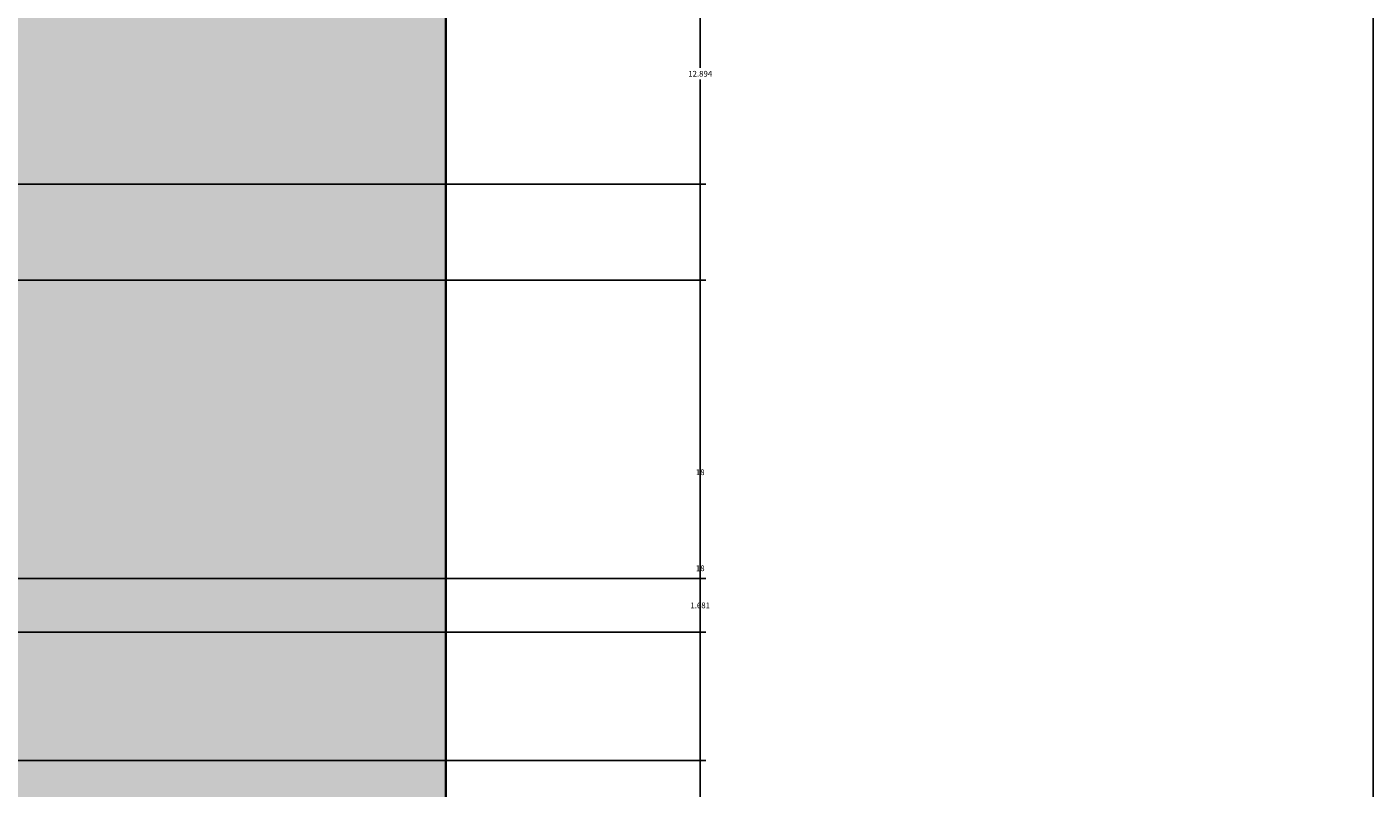
# Model space of a CAD drawing. Units: inches. Extents: x 4508 to 4723, y 847 to 1020.
# Tile 24 of 32: x 4681 to 4723, y 886 to 910. Entities that reach past the tile are written whole.
import ezdxf

# ---------------------------------------------------------------- set-up
doc = ezdxf.new("R2010")
doc.units = ezdxf.units.IN
for name, color, linetype, lineweight in [('A-ANNO-DIMS', 2, 'Continuous', 18), ('A-ANNO-TTLB', 7, 'Continuous', 25), ('A-WALL', 7, 'Continuous', 35), ('A-WALL-PATT', 254, 'Continuous', 13)]:
    doc.layers.add(name, color=color, linetype=linetype, lineweight=lineweight)
doc.styles.get("Standard").update_dxf_attribs({"font": 'arial.ttf'})
doc.dimstyles.get("Standard").update_dxf_attribs({"dimtxt": 0.18, "dimasz": 0.18, "dimexe": 0.18, "dimexo": 0.0625, "dimgap": 0.09, "dimtad": 0, "dimtih": 1, "dimtoh": 1, "dimdec": 4, "dimzin": 0, "dimdsep": 46, "dimtxsty": 'Standard', "dimcen": 0.09, "dimadec": 0, "dimazin": 0, "dimtfac": 1, "dimtdec": 4, "dimtofl": 0, "dimtmove": 0, "dimatfit": 3, "dimfxl": 1, "dimtolj": 1, "dimtzin": 0, "dimarcsym": 0})

# ---------------------------------------------------------------- blocks, each defined once
blk = doc.blocks.new('*D13')
at = {"layer": 'A-ANNO-DIMS', "color": 0, "lineweight": -2, "transparency": 16777216}
for p, q in [((4669.325, 973.916), (4669.325, 866.617)), ((4689.994, 874.684), (4689.994, 866.617)), ((4669.505, 866.797), (4679.264, 866.797)), ((4689.814, 866.797), (4680.054, 866.797))]:
    blk.add_line(p, q, dxfattribs=at)
at = {"layer": 'A-ANNO-DIMS', "color": 0, "lineweight": 9, "transparency": 16777216}
for points in [[(4669.505, 866.827), (4669.505, 866.767), (4669.325, 866.797)], [(4689.814, 866.827), (4689.814, 866.767), (4689.994, 866.797)]]:
    blk.add_solid(points, dxfattribs=at)
at = {"layer": 'Defpoints', "color": 0, "lineweight": 9, "transparency": 16777216}
for p in [(4669.325, 973.978), (4689.994, 874.747), (4689.994, 866.797)]:
    blk.add_point(p, dxfattribs=at)
at = {"layer": 'A-ANNO-DIMS', "color": 0, "transparency": 16777216, "insert": (4679.659, 866.797), "char_height": 0.18, "attachment_point": 5}
blk.add_mtext('\\A1;20.67', dxfattribs=at)
blk = doc.blocks.new('*D18')
at = {"layer": 'A-ANNO-DIMS', "color": 0, "lineweight": -2, "transparency": 16777216}
for p, q in [((4671.119, 901.747), (4702.124, 901.747)), ((4701.944, 901.567), (4701.944, 892.929)), ((4701.944, 883.927), (4701.944, 892.565)), ((4671.869, 883.747), (4702.124, 883.747))]:
    blk.add_line(p, q, dxfattribs=at)
at = {"layer": 'A-ANNO-DIMS', "color": 0, "lineweight": 9, "transparency": 16777216}
for points in [[(4701.914, 901.567), (4701.974, 901.567), (4701.944, 901.747)], [(4701.914, 883.927), (4701.974, 883.927), (4701.944, 883.747)]]:
    blk.add_solid(points, dxfattribs=at)
at = {"layer": 'Defpoints', "color": 0, "lineweight": 9, "transparency": 16777216}
for p in [(4671.056, 901.747), (4701.944, 901.747), (4671.806, 883.747)]:
    blk.add_point(p, dxfattribs=at)
at = {"layer": 'A-ANNO-DIMS', "color": 0, "transparency": 16777216, "insert": (4701.944, 892.747), "char_height": 0.18, "attachment_point": 5}
blk.add_mtext('\\A1;18', dxfattribs=at)
blk = doc.blocks.new('*D19')
at = {"layer": 'A-ANNO-DIMS', "color": 0, "lineweight": -2, "transparency": 16777216}
for p, q in [((4662.233, 914.641), (4702.124, 914.641)), ((4701.944, 914.461), (4701.944, 908.376)), ((4701.944, 901.927), (4701.944, 908.012)), ((4671.119, 901.747), (4702.124, 901.747))]:
    blk.add_line(p, q, dxfattribs=at)
at = {"layer": 'A-ANNO-DIMS', "color": 0, "lineweight": 9, "transparency": 16777216}
for points in [[(4701.914, 914.461), (4701.974, 914.461), (4701.944, 914.641)], [(4701.914, 901.927), (4701.974, 901.927), (4701.944, 901.747)]]:
    blk.add_solid(points, dxfattribs=at)
at = {"layer": 'Defpoints', "color": 0, "lineweight": 9, "transparency": 16777216}
for p in [(4662.171, 914.641), (4701.944, 914.641), (4671.056, 901.747)]:
    blk.add_point(p, dxfattribs=at)
at = {"layer": 'A-ANNO-DIMS', "color": 0, "transparency": 16777216, "insert": (4701.944, 908.194), "char_height": 0.18, "attachment_point": 5}
blk.add_mtext('\\A1;12.894', dxfattribs=at)
blk = doc.blocks.new('*D25')
at = {"layer": 'A-ANNO-DIMS', "color": 0, "lineweight": -2, "transparency": 16777216}
for p, q in [((4658.056, 904.747), (4702.124, 904.747)), ((4701.944, 904.567), (4701.944, 895.929)), ((4701.944, 886.927), (4701.944, 895.565)), ((4658.056, 886.747), (4702.124, 886.747))]:
    blk.add_line(p, q, dxfattribs=at)
at = {"layer": 'A-ANNO-DIMS', "color": 0, "lineweight": 9, "transparency": 16777216}
for points in [[(4701.914, 904.567), (4701.974, 904.567), (4701.944, 904.747)], [(4701.914, 886.927), (4701.974, 886.927), (4701.944, 886.747)]]:
    blk.add_solid(points, dxfattribs=at)
at = {"layer": 'Defpoints', "color": 0, "lineweight": 9, "transparency": 16777216}
for p in [(4657.994, 904.747), (4701.944, 904.747), (4657.994, 886.747)]:
    blk.add_point(p, dxfattribs=at)
at = {"layer": 'A-ANNO-DIMS', "color": 0, "transparency": 16777216, "insert": (4701.944, 895.747), "char_height": 0.18, "attachment_point": 5}
blk.add_mtext('\\A1;18', dxfattribs=at)
blk = doc.blocks.new('*D35')
at = {"layer": 'A-ANNO-DIMS', "color": 0, "lineweight": -2, "transparency": 16777216}
for p, q in [((4625.361, 892.428), (4702.124, 892.428)), ((4701.944, 892.248), (4701.944, 891.769)), ((4701.944, 890.927), (4701.944, 891.405)), ((4625.361, 890.747), (4702.124, 890.747))]:
    blk.add_line(p, q, dxfattribs=at)
at = {"layer": 'A-ANNO-DIMS', "color": 0, "lineweight": 9, "transparency": 16777216}
for points in [[(4701.914, 892.248), (4701.974, 892.248), (4701.944, 892.428)], [(4701.914, 890.927), (4701.974, 890.927), (4701.944, 890.747)]]:
    blk.add_solid(points, dxfattribs=at)
at = {"layer": 'Defpoints', "color": 0, "lineweight": 9, "transparency": 16777216}
for p in [(4625.298, 892.428), (4701.944, 892.428), (4625.298, 890.747)]:
    blk.add_point(p, dxfattribs=at)
at = {"layer": 'A-ANNO-DIMS', "color": 0, "transparency": 16777216, "insert": (4701.944, 891.587), "char_height": 0.18, "attachment_point": 5}
blk.add_mtext('\\A1;1.681', dxfattribs=at)

msp = doc.modelspace()

# ---------------------------------------------------------------- hatches: boundary and pattern name
at = {"layer": 'A-WALL-PATT', "transparency": 33554508}
h = msp.add_hatch(color=256, dxfattribs=at)
h.dxf.hatch_style = 1
h.paths.add_polyline_path([(4661.6706, 954.043, -0.3739004), (4658.5765, 957.6021, -1), (4665.7646, 957.6021, -0.3739004), (4662.6706, 954.043), (4662.6706, 944.4021, -0.2114781), (4670.3062, 945.0869), (4670.3062, 968.0592, -0.4632086), (4663.3246, 973.9783, -0.4632086), (4670.3062, 979.8975), (4670.3062, 994.7469), (4588.9938, 994.7469), (4588.9938, 904.7469), (4657.9938, 904.7469), (4657.9938, 886.7469), (4549.9938, 886.7469), (4549.9938, 878.7469), (4693.9938, 878.7469), (4693.9938, 994.7469), (4671.8062, 994.7469), (4671.8062, 979.4411, -0.2941682), (4675.3246, 973.9783, -0.2941682), (4671.8062, 968.5156), (4671.8062, 944.4278, -0.2741114), (4676.7298, 936.1217, -0.2741114), (4671.8062, 927.8155), (4671.8062, 907.6998, -0.3779645), (4677.0562, 901.7469, -0.3779645), (4671.8062, 895.7939), (4671.8062, 883.7469), (4670.3062, 883.7469), (4670.3062, 895.7939, -0.3779645), (4665.0562, 901.7469, -0.3779645), (4670.3062, 907.6998), (4670.3062, 927.1564, -0.2114781), (4662.6706, 927.8412), (4662.6706, 918.2003, -0.3739004), (4665.7646, 914.6412, -1), (4658.5765, 914.6412, -0.3739004), (4661.6706, 918.2003), (4661.6706, 928.4807, -0.2391825), (4657.7936, 936.1217, -0.2391825), (4661.6706, 943.7626)])

# ---------------------------------------------------------------- linework, layer by layer
at = {"layer": 'A-ANNO-TTLB'}
msp.add_lwpolyline([(4508.3867, 1019.9118), (4722.9774, 1019.9118), (4722.9774, 846.9535), (4508.3867, 846.9535)], close=True, dxfattribs=at)
at = {"layer": 'A-WALL'}
msp.add_line((4693.9938, 994.7469), (4693.9938, 874.7469), dxfattribs=at)

# ---------------------------------------------------------------- dimensions: what is measured, and where the dimension line sits
at = {"layer": 'A-ANNO-DIMS'}
dim = msp.add_linear_dim(base=(4689.9938, 866.7969), p1=(4669.3246, 973.9783), p2=(4689.9938, 874.7469), dimstyle='Standard', override={"dimdec": 2, "dimlfac": 1, "dimrnd": 0, "dimzin": 0, "dimdsep": 46, "dimlunit": 2}, dxfattribs=at)
dim.commit()
dim.dimension.update_dxf_attribs({"geometry": '*D13', "text_midpoint": (4679.6592, 866.7969)})
for base, p1, p2, override, picture, middle in [((4701.9438, 914.6412), (4671.0562, 901.7469), (4662.1706, 914.6412), {"dimdec": 3, "dimlfac": 1, "dimrnd": 0, "dimzin": 0, "dimdsep": 46, "dimlunit": 2}, '*D19', (4701.9438, 908.1941)), ((4701.9438, 904.7469), (4657.9938, 886.7469), (4657.9938, 904.7469), {"dimdec": 0, "dimlfac": 1, "dimrnd": 0, "dimzin": 0, "dimdsep": 46, "dimlunit": 2}, '*D25', (4701.9438, 895.7469)), ((4701.9438, 901.7469), (4671.8062, 883.7469), (4671.0562, 901.7469), {"dimdec": 0, "dimlfac": 1, "dimrnd": 0, "dimzin": 0, "dimdsep": 46, "dimlunit": 2}, '*D18', (4701.9438, 892.7469)), ((4701.9438, 892.4277), (4625.2983, 890.7469), (4625.2983, 892.4277), {"dimdec": 3, "dimlfac": 1, "dimrnd": 0, "dimzin": 0, "dimdsep": 46, "dimlunit": 2}, '*D35', (4701.9438, 891.5873))]:
    dim = msp.add_linear_dim(base=base, p1=p1, p2=p2, angle=90, dimstyle='Standard', override=override, dxfattribs=at)
    dim.commit()
    dim.dimension.update_dxf_attribs({"geometry": picture, "text_midpoint": middle})

doc.saveas('drawing.dxf')
